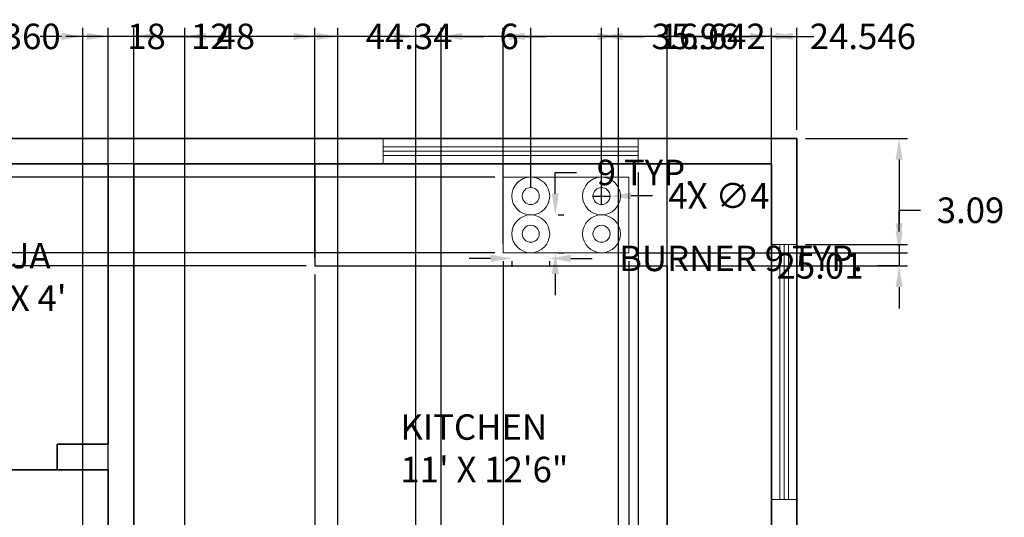
# Model space of a CAD drawing. Units: inches. Extents: x 185 to 668, y 153 to 689.
# Tile 5 of 5: x 420 to 652, y 572 to 689. Entities that reach past the tile are written whole.
import ezdxf

# ---------------------------------------------------------------- set-up
doc = ezdxf.new("R2010")
doc.units = ezdxf.units.IN
doc.header["$MEASUREMENT"] = 0
for name, color, linetype, lineweight in [('A-ANNO-DIMS', 2, 'Continuous', 18), ('A-AREA-IDEN', 7, 'Continuous', 25), ('A-EQPM', 9, 'Continuous', 18), ('A-FLOR-CASE', 8, 'Continuous', 25), ('A-GLAZ', 4, 'Continuous', 18), ('A-WALL', 7, 'Continuous', 35)]:
    doc.layers.add(name, color=color, linetype=linetype, lineweight=lineweight)
doc.styles.get("Standard").update_dxf_attribs({"font": 'arial.ttf'})
doc.dimstyles.get("Standard").update_dxf_attribs({"dimtxt": 6, "dimasz": 5, "dimexe": 2, "dimexo": 2, "dimgap": 4, "dimtad": 0, "dimtih": 1, "dimtoh": 1, "dimdec": 0, "dimzin": 0, "dimdsep": 46, "dimlunit": 3, "dimtxsty": 'Standard', "dimcen": 2, "dimadec": 0, "dimazin": 0, "dimtfac": 1, "dimtdec": 0, "dimtofl": 0, "dimtmove": 0, "dimatfit": 3, "dimfxl": 1, "dimtolj": 1, "dimtzin": 0, "dimarcsym": 0})

# ---------------------------------------------------------------- blocks, each defined once
blk = doc.blocks.new('WINDOW-60')
for p, q in [((2, 60), (0, 60)), ((2, 60), (2, 0)), ((4, 60), (2, 60)), ((3, 0), (3, 60)), ((4, 0), (4, 60)), ((4, 60), (6, 60)), ((6, 0), (0, 0)), ((2, 0), (0, 0)), ((2, 0), (4, 0)), ((4, 0), (6, 0))]:
    blk.add_line(p, q)
blk = doc.blocks.new('BURNER-COOKTOP')
for radius in [4.45, 2]:
    blk.add_circle((4.45, 4.45), radius)
blk = doc.blocks.new('*D13')
at = {"layer": 'A-ANNO-DIMS', "color": 0, "lineweight": -2, "transparency": 16777216}
for p, q in [((530.97, 633.14), (525.97, 633.14)), ((535.97, 632.47), (535.97, 631.14)), ((544.86, 632.47), (544.86, 631.14)), ((549.86, 633.14), (554.86, 633.14))]:
    blk.add_line(p, q, dxfattribs=at)
at = {"layer": 'A-ANNO-DIMS', "color": 0, "transparency": 16777216}
for points in [[(530.97, 633.97), (530.97, 632.31), (535.97, 633.14)], [(549.86, 633.97), (549.86, 632.31), (544.86, 633.14)]]:
    blk.add_solid(points, dxfattribs=at)
at = {"layer": 'Defpoints', "color": 0, "transparency": 16777216}
for p in [(535.97, 634.47), (544.86, 634.47), (544.86, 633.14)]:
    blk.add_point(p, dxfattribs=at)
at = {"layer": 'A-ANNO-DIMS', "color": 0, "transparency": 16777216, "insert": (589.86, 633.14), "char_height": 6, "attachment_point": 5}
blk.add_mtext('\\A1;BURNER 9 TYP.', dxfattribs=at)
blk = doc.blocks.new('*D14')
at = {"layer": 'A-ANNO-DIMS', "color": 0, "lineweight": -2, "transparency": 16777216}
for p, q in [((546.2, 648.37), (546.2, 653.37)), ((546.2, 653.37), (551.2, 653.37)), ((546.86, 643.37), (548.2, 643.37)), ((546.86, 634.47), (548.2, 634.47)), ((546.2, 629.47), (546.2, 624.47))]:
    blk.add_line(p, q, dxfattribs=at)
at = {"layer": 'A-ANNO-DIMS', "color": 0, "transparency": 16777216}
for points in [[(545.36, 648.37), (547.03, 648.37), (546.2, 643.37)], [(545.36, 629.47), (547.03, 629.47), (546.2, 634.47)]]:
    blk.add_solid(points, dxfattribs=at)
at = {"layer": 'Defpoints', "color": 0, "transparency": 16777216}
for p in [(544.86, 643.37), (546.2, 643.37), (544.86, 634.47)]:
    blk.add_point(p, dxfattribs=at)
at = {"layer": 'A-ANNO-DIMS', "color": 0, "transparency": 16777216, "insert": (567.47, 653.37), "char_height": 6, "attachment_point": 5}
blk.add_mtext('\\A1;9 TYP.', dxfattribs=at)
blk = doc.blocks.new('*D25')
at = {"layer": 'A-ANNO-DIMS', "color": 0, "lineweight": -2, "transparency": 16777216}
for p, q in [((243.04, 663.38), (243.04, 687.4)), ((603.04, 663.38), (603.04, 687.4)), ((248.04, 685.4), (412.42, 685.4)), ((598.04, 685.4), (433.66, 685.4))]:
    blk.add_line(p, q, dxfattribs=at)
at = {"layer": 'A-ANNO-DIMS', "color": 0, "transparency": 16777216}
for points in [[(248.04, 686.23), (248.04, 684.56), (243.04, 685.4)], [(598.04, 686.23), (598.04, 684.56), (603.04, 685.4)]]:
    blk.add_solid(points, dxfattribs=at)
at = {"layer": 'Defpoints', "color": 0, "transparency": 16777216}
for p in [(603.04, 685.4), (243.04, 661.38), (603.04, 661.38)]:
    blk.add_point(p, dxfattribs=at)
at = {"layer": 'A-ANNO-DIMS', "color": 0, "transparency": 16777216, "insert": (423.04, 685.4), "char_height": 6, "attachment_point": 5}
blk.add_mtext('\\A1;360', dxfattribs=at)
blk = doc.blocks.new('*D31')
at = {"layer": 'A-ANNO-DIMS', "color": 0, "lineweight": -2, "transparency": 16777216}
for p, q in [((605.04, 661.38), (629.06, 661.38)), ((627.06, 656.38), (627.06, 641.37)), ((605.04, 636.37), (629.06, 636.37)), ((627.06, 636.37), (627.06, 631.37)), ((627.06, 631.37), (622.06, 631.37))]:
    blk.add_line(p, q, dxfattribs=at)
at = {"layer": 'A-ANNO-DIMS', "color": 0, "transparency": 16777216}
for points in [[(626.23, 656.38), (627.89, 656.38), (627.06, 661.38)], [(626.23, 641.37), (627.89, 641.37), (627.06, 636.37)]]:
    blk.add_solid(points, dxfattribs=at)
at = {"layer": 'Defpoints', "color": 0, "transparency": 16777216}
for p in [(603.04, 661.38), (603.04, 636.37), (627.06, 636.37)]:
    blk.add_point(p, dxfattribs=at)
at = {"layer": 'A-ANNO-DIMS', "color": 0, "transparency": 16777216, "insert": (608.46, 631.37), "char_height": 6, "attachment_point": 5}
blk.add_mtext('\\A1;25.01', dxfattribs=at)
blk = doc.blocks.new('*D33')
at = {"layer": 'A-ANNO-DIMS', "color": 0, "lineweight": -2, "transparency": 16777216}
for p, q in [((565.69, 653.38), (565.69, 155.36)), ((597.04, 653.38), (597.04, 155.36)), ((560.69, 157.36), (555.69, 157.36)), ((602.04, 157.36), (607.04, 157.36))]:
    blk.add_line(p, q, dxfattribs=at)
at = {"layer": 'A-ANNO-DIMS', "color": 0, "transparency": 16777216}
for points in [[(560.69, 158.19), (560.69, 156.53), (565.69, 157.36)], [(602.04, 158.19), (602.04, 156.53), (597.04, 157.36)]]:
    blk.add_solid(points, dxfattribs=at)
at = {"layer": 'Defpoints', "color": 0, "transparency": 16777216}
for p in [(565.69, 655.38), (597.04, 655.38), (597.04, 157.36)]:
    blk.add_point(p, dxfattribs=at)
at = {"layer": 'A-ANNO-DIMS', "color": 0, "transparency": 16777216, "insert": (581.37, 157.36), "char_height": 6, "attachment_point": 5}
blk.add_mtext('\\A1;31.35', dxfattribs=at)
blk = doc.blocks.new('*D42')
at = {"layer": 'A-ANNO-DIMS', "color": 0, "lineweight": -2, "transparency": 16777216}
for p, q in [((487.63, 655.38), (217.02, 655.38)), ((219.02, 650.38), (219.02, 636.38)), ((487.63, 631.38), (217.02, 631.38)), ((219.02, 631.38), (219.02, 626.38)), ((219.02, 626.38), (214.02, 626.38))]:
    blk.add_line(p, q, dxfattribs=at)
at = {"layer": 'A-ANNO-DIMS', "color": 0, "transparency": 16777216}
for points in [[(218.19, 650.38), (219.86, 650.38), (219.02, 655.38)], [(218.19, 636.38), (219.86, 636.38), (219.02, 631.38)]]:
    blk.add_solid(points, dxfattribs=at)
at = {"layer": 'Defpoints', "color": 0, "transparency": 16777216}
for p in [(489.63, 655.38), (219.02, 631.38), (489.63, 631.38)]:
    blk.add_point(p, dxfattribs=at)
at = {"layer": 'A-ANNO-DIMS', "color": 0, "transparency": 16777216, "insert": (205.69, 626.38), "char_height": 6, "attachment_point": 5}
blk.add_mtext('\\A1;24', dxfattribs=at)
blk = doc.blocks.new('*D43')
at = {"layer": 'A-ANNO-DIMS', "color": 0, "lineweight": -2, "transparency": 16777216}
for p, q in [((489.63, 629.38), (489.63, 155.36)), ((572.5, 629.38), (572.5, 155.36)), ((494.63, 157.36), (516.94, 157.36)), ((567.5, 157.36), (545.19, 157.36))]:
    blk.add_line(p, q, dxfattribs=at)
at = {"layer": 'A-ANNO-DIMS', "color": 0, "transparency": 16777216}
for points in [[(494.63, 158.19), (494.63, 156.53), (489.63, 157.36)], [(567.5, 158.19), (567.5, 156.53), (572.5, 157.36)]]:
    blk.add_solid(points, dxfattribs=at)
at = {"layer": 'Defpoints', "color": 0, "transparency": 16777216}
for p in [(489.63, 631.38), (572.5, 631.38), (572.5, 157.36)]:
    blk.add_point(p, dxfattribs=at)
at = {"layer": 'A-ANNO-DIMS', "color": 0, "transparency": 16777216, "insert": (531.06, 157.36), "char_height": 6, "attachment_point": 5}
blk.add_mtext('\\A1;82.86', dxfattribs=at)
blk = doc.blocks.new('*D44')
at = {"layer": 'A-ANNO-DIMS', "color": 0, "lineweight": -2, "transparency": 16777216}
for p, q in [((447.04, 519.38), (447.04, 687.4)), ((495.04, 525.38), (495.04, 687.4)), ((452.04, 685.4), (462.62, 685.4)), ((490.04, 685.4), (479.47, 685.4))]:
    blk.add_line(p, q, dxfattribs=at)
at = {"layer": 'A-ANNO-DIMS', "color": 0, "transparency": 16777216}
for points in [[(452.04, 686.23), (452.04, 684.56), (447.04, 685.4)], [(490.04, 686.23), (490.04, 684.56), (495.04, 685.4)]]:
    blk.add_solid(points, dxfattribs=at)
at = {"layer": 'Defpoints', "color": 0, "transparency": 16777216}
for p in [(495.04, 685.4), (495.04, 523.38), (447.04, 517.38)]:
    blk.add_point(p, dxfattribs=at)
at = {"layer": 'A-ANNO-DIMS', "color": 0, "transparency": 16777216, "insert": (471.04, 685.4), "char_height": 6, "attachment_point": 5}
blk.add_mtext('\\A1;48', dxfattribs=at)
blk = doc.blocks.new('*D45')
at = {"layer": 'A-ANNO-DIMS', "color": 0, "lineweight": -2, "transparency": 16777216}
for p, q in [((435.04, 417.38), (435.04, 687.4)), ((447.04, 417.38), (447.04, 687.4)), ((430.04, 685.4), (425.04, 685.4)), ((452.04, 685.4), (457.04, 685.4))]:
    blk.add_line(p, q, dxfattribs=at)
at = {"layer": 'A-ANNO-DIMS', "color": 0, "transparency": 16777216}
for points in [[(430.04, 686.23), (430.04, 684.56), (435.04, 685.4)], [(452.04, 686.23), (452.04, 684.56), (447.04, 685.4)]]:
    blk.add_solid(points, dxfattribs=at)
at = {"layer": 'Defpoints', "color": 0, "transparency": 16777216}
for p in [(447.04, 685.4), (435.04, 415.38), (447.04, 415.38)]:
    blk.add_point(p, dxfattribs=at)
at = {"layer": 'A-ANNO-DIMS', "color": 0, "transparency": 16777216, "insert": (465.03, 685.4), "char_height": 6, "attachment_point": 5}
blk.add_mtext('\\A1;12', dxfattribs=at)
blk = doc.blocks.new('*D46')
at = {"layer": 'A-ANNO-DIMS', "color": 0, "lineweight": -2, "transparency": 16777216}
for p, q in [((513.35, 417.38), (513.35, 687.4)), ((519.35, 417.38), (519.35, 687.4)), ((508.35, 685.4), (503.35, 685.4)), ((524.35, 685.4), (529.35, 685.4))]:
    blk.add_line(p, q, dxfattribs=at)
at = {"layer": 'A-ANNO-DIMS', "color": 0, "transparency": 16777216}
for points in [[(508.35, 686.23), (508.35, 684.56), (513.35, 685.4)], [(524.35, 686.23), (524.35, 684.56), (519.35, 685.4)]]:
    blk.add_solid(points, dxfattribs=at)
at = {"layer": 'Defpoints', "color": 0, "transparency": 16777216}
for p in [(519.35, 685.4), (513.35, 415.38), (519.35, 415.38)]:
    blk.add_point(p, dxfattribs=at)
at = {"layer": 'A-ANNO-DIMS', "color": 0, "transparency": 16777216, "insert": (535.33, 685.4), "char_height": 6, "attachment_point": 5}
blk.add_mtext('\\A1;6', dxfattribs=at)
blk = doc.blocks.new('*D49')
at = {"layer": 'A-ANNO-DIMS', "color": 0, "lineweight": -2, "transparency": 16777216}
for p, q in [((572.5, 525.38), (572.5, 687.4)), ((597.04, 525.38), (597.04, 687.4)), ((577.5, 685.4), (592.04, 685.4)), ((597.04, 685.4), (602.04, 685.4))]:
    blk.add_line(p, q, dxfattribs=at)
at = {"layer": 'A-ANNO-DIMS', "color": 0, "transparency": 16777216}
for points in [[(577.5, 686.23), (577.5, 684.56), (572.5, 685.4)], [(592.04, 686.23), (592.04, 684.56), (597.04, 685.4)]]:
    blk.add_solid(points, dxfattribs=at)
at = {"layer": 'Defpoints', "color": 0, "transparency": 16777216}
for p in [(597.04, 685.4), (572.5, 523.38), (597.04, 523.38)]:
    blk.add_point(p, dxfattribs=at)
at = {"layer": 'A-ANNO-DIMS', "color": 0, "transparency": 16777216, "insert": (618.54, 685.4), "char_height": 6, "attachment_point": 5}
blk.add_mtext('\\A1;24.546', dxfattribs=at)
blk = doc.blocks.new('*D52')
at = {"layer": 'A-ANNO-DIMS', "color": 0, "lineweight": -2, "transparency": 16777216}
for p, q in [((441.04, 344.34), (441.04, 687.4)), ((459.04, 344.34), (459.04, 687.4)), ((436.04, 685.4), (431.04, 685.4)), ((464.04, 685.4), (469.04, 685.4))]:
    blk.add_line(p, q, dxfattribs=at)
at = {"layer": 'A-ANNO-DIMS', "color": 0, "transparency": 16777216}
for points in [[(436.04, 686.23), (436.04, 684.56), (441.04, 685.4)], [(464.04, 686.23), (464.04, 684.56), (459.04, 685.4)]]:
    blk.add_solid(points, dxfattribs=at)
at = {"layer": 'Defpoints', "color": 0, "transparency": 16777216}
for p in [(459.04, 685.4), (441.04, 342.34), (459.04, 342.34)]:
    blk.add_point(p, dxfattribs=at)
at = {"layer": 'A-ANNO-DIMS', "color": 0, "transparency": 16777216, "insert": (450.04, 685.4), "char_height": 6, "attachment_point": 5}
blk.add_mtext('\\A1;18', dxfattribs=at)
blk = doc.blocks.new('*D62')
at = {"layer": 'A-ANNO-DIMS', "color": 0, "lineweight": -2, "transparency": 16777216}
for p, q in [((533.97, 632.47), (533.97, 155.36)), ((563.51, 632.47), (563.51, 155.36)), ((538.97, 157.36), (558.51, 157.36)), ((563.51, 157.36), (568.51, 157.36))]:
    blk.add_line(p, q, dxfattribs=at)
at = {"layer": 'A-ANNO-DIMS', "color": 0, "transparency": 16777216}
for points in [[(538.97, 158.19), (538.97, 156.53), (533.97, 157.36)], [(558.51, 158.19), (558.51, 156.53), (563.51, 157.36)]]:
    blk.add_solid(points, dxfattribs=at)
at = {"layer": 'Defpoints', "color": 0, "transparency": 16777216}
for p in [(533.97, 634.47), (563.51, 634.47), (563.51, 157.36)]:
    blk.add_point(p, dxfattribs=at)
at = {"layer": 'A-ANNO-DIMS', "color": 0, "transparency": 16777216, "insert": (585.01, 157.36), "char_height": 6, "attachment_point": 5}
blk.add_mtext('\\A1;29.536', dxfattribs=at)
blk = doc.blocks.new('*D63')
at = {"layer": 'A-ANNO-DIMS', "color": 0, "lineweight": -2, "transparency": 16777216}
for p, q in [((219.02, 657.26), (219.02, 662.26)), ((531.97, 652.26), (217.02, 652.26)), ((531.97, 634.47), (217.02, 634.47)), ((219.02, 629.47), (219.02, 624.47))]:
    blk.add_line(p, q, dxfattribs=at)
at = {"layer": 'A-ANNO-DIMS', "color": 0, "transparency": 16777216}
for points in [[(218.19, 657.26), (219.86, 657.26), (219.02, 652.26)], [(218.19, 629.47), (219.86, 629.47), (219.02, 634.47)]]:
    blk.add_solid(points, dxfattribs=at)
at = {"layer": 'Defpoints', "color": 0, "transparency": 16777216}
for p in [(219.02, 652.26), (533.97, 652.26), (533.97, 634.47)]:
    blk.add_point(p, dxfattribs=at)
at = {"layer": 'A-ANNO-DIMS', "color": 0, "transparency": 16777216, "insert": (219.02, 643.37), "char_height": 6, "attachment_point": 5}
blk.add_mtext('\\A1;17.79', dxfattribs=at)
blk = doc.blocks.new('*D64')
at = {"layer": 'A-ANNO-DIMS', "color": 0, "lineweight": -2, "transparency": 16777216}
for p, q in [((540.42, 649.81), (540.42, 687.4)), ((557.06, 649.81), (557.06, 687.4)), ((535.42, 685.4), (530.42, 685.4)), ((562.06, 685.4), (567.06, 685.4))]:
    blk.add_line(p, q, dxfattribs=at)
at = {"layer": 'A-ANNO-DIMS', "color": 0, "transparency": 16777216}
for points in [[(535.42, 686.23), (535.42, 684.56), (540.42, 685.4)], [(562.06, 686.23), (562.06, 684.56), (557.06, 685.4)]]:
    blk.add_solid(points, dxfattribs=at)
at = {"layer": 'Defpoints', "color": 0, "transparency": 16777216}
for p in [(557.06, 685.4), (540.42, 647.81), (557.06, 647.81)]:
    blk.add_point(p, dxfattribs=at)
at = {"layer": 'A-ANNO-DIMS', "color": 0, "transparency": 16777216, "insert": (583.2, 685.4), "char_height": 6, "attachment_point": 5}
blk.add_mtext('\\A1;16.642', dxfattribs=at)
blk = doc.blocks.new('*D66')
at = {"layer": 'A-ANNO-DIMS', "color": 0, "lineweight": -2, "transparency": 16777216}
for p, q in [((219.02, 569.09), (219.02, 574.09)), ((219.02, 574.09), (224.02, 574.09)), ((578.09, 569.09), (217.02, 569.09)), ((219.02, 549.77), (219.02, 564.09)), ((578.09, 544.77), (217.02, 544.77))]:
    blk.add_line(p, q, dxfattribs=at)
at = {"layer": 'A-ANNO-DIMS', "color": 0, "transparency": 16777216}
for points in [[(218.19, 564.09), (219.86, 564.09), (219.02, 569.09)], [(218.19, 549.77), (219.86, 549.77), (219.02, 544.77)]]:
    blk.add_solid(points, dxfattribs=at)
at = {"layer": 'Defpoints', "color": 0, "transparency": 16777216}
for p in [(219.02, 569.09), (580.09, 569.09), (580.09, 544.77)]:
    blk.add_point(p, dxfattribs=at)
at = {"layer": 'A-ANNO-DIMS', "color": 0, "transparency": 16777216, "insert": (240.55, 574.09), "char_height": 6, "attachment_point": 5}
blk.add_mtext('\\A1;24.315', dxfattribs=at)
blk = doc.blocks.new('*D67')
at = {"layer": 'A-ANNO-DIMS', "color": 0, "lineweight": -2, "transparency": 16777216}
for p, q in [((489.63, 633.38), (489.63, 687.4)), ((533.97, 636.47), (533.97, 687.4)), ((484.63, 685.4), (479.63, 685.4)), ((538.97, 685.4), (543.97, 685.4))]:
    blk.add_line(p, q, dxfattribs=at)
at = {"layer": 'A-ANNO-DIMS', "color": 0, "transparency": 16777216}
for points in [[(484.63, 686.23), (484.63, 684.56), (489.63, 685.4)], [(538.97, 686.23), (538.97, 684.56), (533.97, 685.4)]]:
    blk.add_solid(points, dxfattribs=at)
at = {"layer": 'Defpoints', "color": 0, "transparency": 16777216}
for p in [(533.97, 685.4), (533.97, 634.47), (489.63, 631.38)]:
    blk.add_point(p, dxfattribs=at)
at = {"layer": 'A-ANNO-DIMS', "color": 0, "transparency": 16777216, "insert": (511.8, 685.4), "char_height": 6, "attachment_point": 5}
blk.add_mtext('\\A1;44.34', dxfattribs=at)
blk = doc.blocks.new('*D68')
at = {"layer": 'A-ANNO-DIMS', "color": 0, "lineweight": -2, "transparency": 16777216}
for p, q in [((627.06, 639.47), (627.06, 644.47)), ((627.06, 644.47), (632.06, 644.47)), ((565.51, 634.47), (629.06, 634.47)), ((574.5, 631.38), (629.06, 631.38)), ((627.06, 626.38), (627.06, 621.38))]:
    blk.add_line(p, q, dxfattribs=at)
at = {"layer": 'A-ANNO-DIMS', "color": 0, "transparency": 16777216}
for points in [[(626.23, 639.47), (627.89, 639.47), (627.06, 634.47)], [(626.23, 626.38), (627.89, 626.38), (627.06, 631.38)]]:
    blk.add_solid(points, dxfattribs=at)
at = {"layer": 'Defpoints', "color": 0, "transparency": 16777216}
for p in [(563.51, 634.47), (627.06, 634.47), (572.5, 631.38)]:
    blk.add_point(p, dxfattribs=at)
at = {"layer": 'A-ANNO-DIMS', "color": 0, "transparency": 16777216, "insert": (643.86, 644.47), "char_height": 6, "attachment_point": 5}
blk.add_mtext('\\A1;3.09', dxfattribs=at)
blk = doc.blocks.new('*D74')
at = {"layer": 'A-ANNO-DIMS', "color": 0, "lineweight": -2, "transparency": 16777216}
for p, q in [((561.08, 272.34), (561.08, 687.4)), ((597.04, 267.38), (597.04, 687.4)), ((556.08, 685.4), (551.08, 685.4)), ((602.04, 685.4), (607.04, 685.4))]:
    blk.add_line(p, q, dxfattribs=at)
at = {"layer": 'A-ANNO-DIMS', "color": 0, "transparency": 16777216}
for points in [[(556.08, 686.23), (556.08, 684.56), (561.08, 685.4)], [(602.04, 686.23), (602.04, 684.56), (597.04, 685.4)]]:
    blk.add_solid(points, dxfattribs=at)
at = {"layer": 'Defpoints', "color": 0, "transparency": 16777216}
for p in [(597.04, 685.4), (561.08, 270.34), (597.04, 265.38)]:
    blk.add_point(p, dxfattribs=at)
at = {"layer": 'A-ANNO-DIMS', "color": 0, "transparency": 16777216, "insert": (579.06, 685.4), "char_height": 6, "attachment_point": 5}
blk.add_mtext('\\A1;35.96', dxfattribs=at)
blk = doc.blocks.new('*D79')
at = {"layer": 'A-ANNO-DIMS', "color": 0, "lineweight": -2, "transparency": 16777216}
for p, q in [((557.06, 645.81), (557.06, 649.81)), ((555.06, 647.81), (559.06, 647.81)), ((569.06, 647.85), (564.06, 647.83))]:
    blk.add_line(p, q, dxfattribs=at)
at = {"layer": 'A-ANNO-DIMS', "color": 0, "transparency": 16777216}
blk.add_solid([(564.06, 648.67), (564.06, 647), (559.06, 647.82)], dxfattribs=at)
at = {"layer": 'Defpoints', "color": 0, "transparency": 16777216}
for p in [(555.06, 647.81), (559.06, 647.82)]:
    blk.add_point(p, dxfattribs=at)
at = {"layer": 'A-ANNO-DIMS', "color": 0, "transparency": 16777216, "insert": (584.68, 647.85), "char_height": 6, "attachment_point": 5}
blk.add_mtext('\\A1;4X ∅4', dxfattribs=at)

msp = doc.modelspace()

# ---------------------------------------------------------------- linework, layer by layer
at = {"layer": 'A-EQPM'}
msp.add_lwpolyline([(533.9695, 652.262), (563.5058, 652.262), (563.5058, 634.4736), (533.9695, 634.4736)], close=True, dxfattribs=at)
at = {"layer": 'A-FLOR-CASE'}
for p, q in [((489.6328, 655.3789), (489.6328, 631.3789)), ((489.6328, 631.3789), (572.4952, 631.3789)), ((572.4952, 631.3789), (572.4952, 523.3789))]:
    msp.add_line(p, q, dxfattribs=at)
at = {"layer": 'A-WALL'}
for p, q in [((603.041, 661.3789), (243.041, 661.3789)), ((603.041, 181.3789), (603.041, 661.3789)), ((441.041, 655.3789), (393.041, 655.3789)), ((441.041, 655.3789), (441.041, 589.3789)), ((447.041, 655.3789), (447.041, 523.3789)), ((597.041, 655.3789), (447.041, 655.3789)), ((597.041, 655.3789), (597.041, 523.3789)), ((441.041, 589.3789), (429.041, 589.3789)), ((429.041, 589.3789), (429.041, 583.3789)), ((429.041, 583.3789), (393.041, 583.3789)), ((441.041, 583.3789), (429.041, 583.3789)), ((441.041, 583.3789), (441.041, 517.3789))]:
    msp.add_line(p, q, dxfattribs=at)

# ---------------------------------------------------------------- block references
at = {"layer": 'A-EQPM'}
for p in [(535.969, 643.368), (552.6112, 643.368), (535.969, 634.4738), (552.6112, 634.4738)]:
    msp.add_blockref('BURNER-COOKTOP', p, dxfattribs=at)
at = {"layer": 'A-GLAZ'}
for p, rotation in [((565.6924, 655.379), 90.00000000000055), ((603.0409, 636.3702), 180)]:
    msp.add_blockref('WINDOW-60', p, dxfattribs=dict(at, rotation=rotation))

# ---------------------------------------------------------------- texts
at = {"layer": 'A-AREA-IDEN', "char_height": 6, "attachment_point": 1}
for s, insert in [('POOJA\\P5\'6" X 4\'', (400.7984, 636.7874)), ('KITCHEN\\P11\' X 12\'6"', (509.7628, 596.44))]:
    msp.add_mtext_dynamic_manual_height_columns(s, width=69.605686, gutter_width=1, heights=[0], dxfattribs=dict(at, insert=insert))

# ---------------------------------------------------------------- dimensions: what is measured, and where the dimension line sits
at = {"layer": 'A-ANNO-DIMS'}
for base, p1, p2, override, picture, middle in [((603.041, 685.3964), (243.041, 661.3789), (603.041, 661.3789), {"dimdec": 0, "dimlfac": 1, "dimrnd": 0, "dimzin": 0, "dimdsep": 46, "dimlunit": 2}, '*D25', (423.041, 685.3964)), ((447.041, 685.3964), (435.041, 415.3789), (447.041, 415.3789), {"dimdec": 0, "dimlfac": 1, "dimrnd": 0, "dimzin": 0, "dimdsep": 46, "dimlunit": 2}, '*D45', (465.0253, 685.3964)), ((459.041, 685.3964), (441.041, 342.3357), (459.041, 342.3357), {"dimdec": 0, "dimlfac": 1, "dimrnd": 0, "dimzin": 0, "dimdsep": 46, "dimlunit": 2}, '*D52', (450.041, 685.3964)), ((495.041, 685.3964), (447.041, 517.3789), (495.041, 523.3789), {"dimdec": 0, "dimlfac": 1, "dimrnd": 0, "dimzin": 0, "dimdsep": 46, "dimlunit": 2}, '*D44', (471.041, 685.3964)), ((533.9695, 685.3964), (489.6328, 631.3789), (533.9695, 634.4736), {"dimdec": 2, "dimlfac": 1, "dimrnd": 0, "dimzin": 0, "dimdsep": 46, "dimlunit": 2}, '*D67', (511.8011, 685.3964)), ((519.3502, 685.3964), (513.3502, 415.3789), (519.3502, 415.3789), {"dimdec": 0, "dimlfac": 1, "dimrnd": 0, "dimzin": 0, "dimdsep": 46, "dimlunit": 2}, '*D46', (535.3311, 685.3964)), ((557.0587, 685.3964), (540.4166, 647.8149), (557.0587, 647.8149), {"dimdec": 3, "dimlfac": 1, "dimrnd": 0, "dimzin": 0, "dimdsep": 46, "dimlunit": 2}, '*D64', (583.1999, 685.3964)), ((597.041, 685.3964), (561.0793, 270.3357), (597.041, 265.3789), {"dimdec": 2, "dimlfac": 1, "dimrnd": 0, "dimzin": 0, "dimdsep": 46, "dimlunit": 2}, '*D74', (579.0601, 685.3964)), ((597.041, 685.3964), (572.4952, 523.3789), (597.041, 523.3789), {"dimdec": 3, "dimlfac": 1, "dimrnd": 0, "dimzin": 0, "dimdsep": 46, "dimlunit": 2}, '*D49', (618.5444, 685.3964)), ((597.041, 157.3614), (565.6925, 655.3789), (597.041, 655.3789), {"dimdec": 2, "dimlfac": 1, "dimrnd": 0, "dimzin": 0, "dimdsep": 46, "dimlunit": 2}, '*D33', (581.3667, 157.3614)), ((563.5058, 157.3614), (533.9695, 634.4736), (563.5058, 634.4736), {"dimdec": 3, "dimlfac": 1, "dimrnd": 0, "dimzin": 0, "dimdsep": 46, "dimlunit": 2}, '*D62', (585.0092, 157.3614)), ((572.4952, 157.3614), (489.6328, 631.3789), (572.4952, 631.3789), {"dimdec": 2, "dimlfac": 1, "dimrnd": 0, "dimzin": 0, "dimdsep": 46, "dimlunit": 2}, '*D43', (531.064, 157.3614))]:
    dim = msp.add_linear_dim(base=base, p1=p1, p2=p2, dimstyle='Standard', override=override, dxfattribs=at)
    dim.commit()
    dim.dimension.update_dxf_attribs({"geometry": picture, "text_midpoint": middle})
for base, p1, p2, override, picture, middle in [((219.0235, 652.262), (533.9695, 634.4736), (533.9695, 652.262), {"dimdec": 2, "dimlfac": 1, "dimrnd": 0, "dimzin": 0, "dimdsep": 46, "dimlunit": 2}, '*D63', (219.0235, 643.3678)), ((627.0585, 636.3704), (603.041, 661.3789), (603.041, 636.3704), {"dimdec": 2, "dimlfac": 1, "dimrnd": 0, "dimzin": 0, "dimdsep": 46, "dimlunit": 2}, '*D31', (608.463, 631.3704)), ((219.0235, 631.3789), (489.6328, 655.3789), (489.6328, 631.3789), {"dimdec": 0, "dimlfac": 1, "dimrnd": 0, "dimzin": 0, "dimdsep": 46, "dimlunit": 2}, '*D42', (205.6872, 626.3789)), ((627.0585, 634.4736), (572.4952, 631.3789), (563.5058, 634.4736), {"dimdec": 2, "dimlfac": 1, "dimrnd": 0, "dimzin": 0, "dimdsep": 46, "dimlunit": 2}, '*D68', (643.8552, 644.4736)), ((219.0235, 569.0859), (580.0867, 544.7709), (580.0867, 569.0859), {"dimdec": 3, "dimlfac": 1, "dimrnd": 0, "dimzin": 0, "dimdsep": 46, "dimlunit": 2}, '*D66', (240.5514, 574.0859))]:
    dim = msp.add_linear_dim(base=base, p1=p1, p2=p2, angle=90, dimstyle='Standard', override=override, dxfattribs=at)
    dim.commit()
    dim.dimension.update_dxf_attribs({"geometry": picture, "text_midpoint": middle})
dim = msp.add_linear_dim(base=(546.1978, 643.3678), p1=(544.8637, 634.4736), p2=(544.8637, 643.3678), angle=90, text='<> TYP.', dimstyle='Standard', override={"dimdec": 0, "dimlfac": 1, "dimrnd": 0, "dimzin": 0, "dimdsep": 46, "dimlunit": 2}, dxfattribs=at)
dim.commit()
dim.dimension.update_dxf_attribs({"geometry": '*D14', "text_midpoint": (567.4699, 653.3678)})
dim = msp.add_diameter_dim_2p(p1=(555.0587, 647.8098), p2=(559.0587, 647.82), text='4X <>', dimstyle='Standard', override={"dimdec": 0, "dimlfac": 1, "dimrnd": 0, "dimzin": 0, "dimdsep": 46, "dimlunit": 2}, dxfattribs=at)
dim.commit()
dim.dimension.update_dxf_attribs({"geometry": '*D79', "text_midpoint": (569.0587, 647.8454), "dimtype": 163})
dim = msp.add_linear_dim(base=(544.8637, 633.1395), p1=(535.9695, 634.4736), p2=(544.8637, 634.4736), text='BURNER <> TYP.', dimstyle='Standard', override={"dimdec": 0, "dimlfac": 1, "dimrnd": 0, "dimzin": 0, "dimdsep": 46, "dimlunit": 2}, dxfattribs=at)
dim.commit()
dim.dimension.update_dxf_attribs({"geometry": '*D13', "text_midpoint": (589.8643, 633.1395)})

doc.saveas('drawing.dxf')
